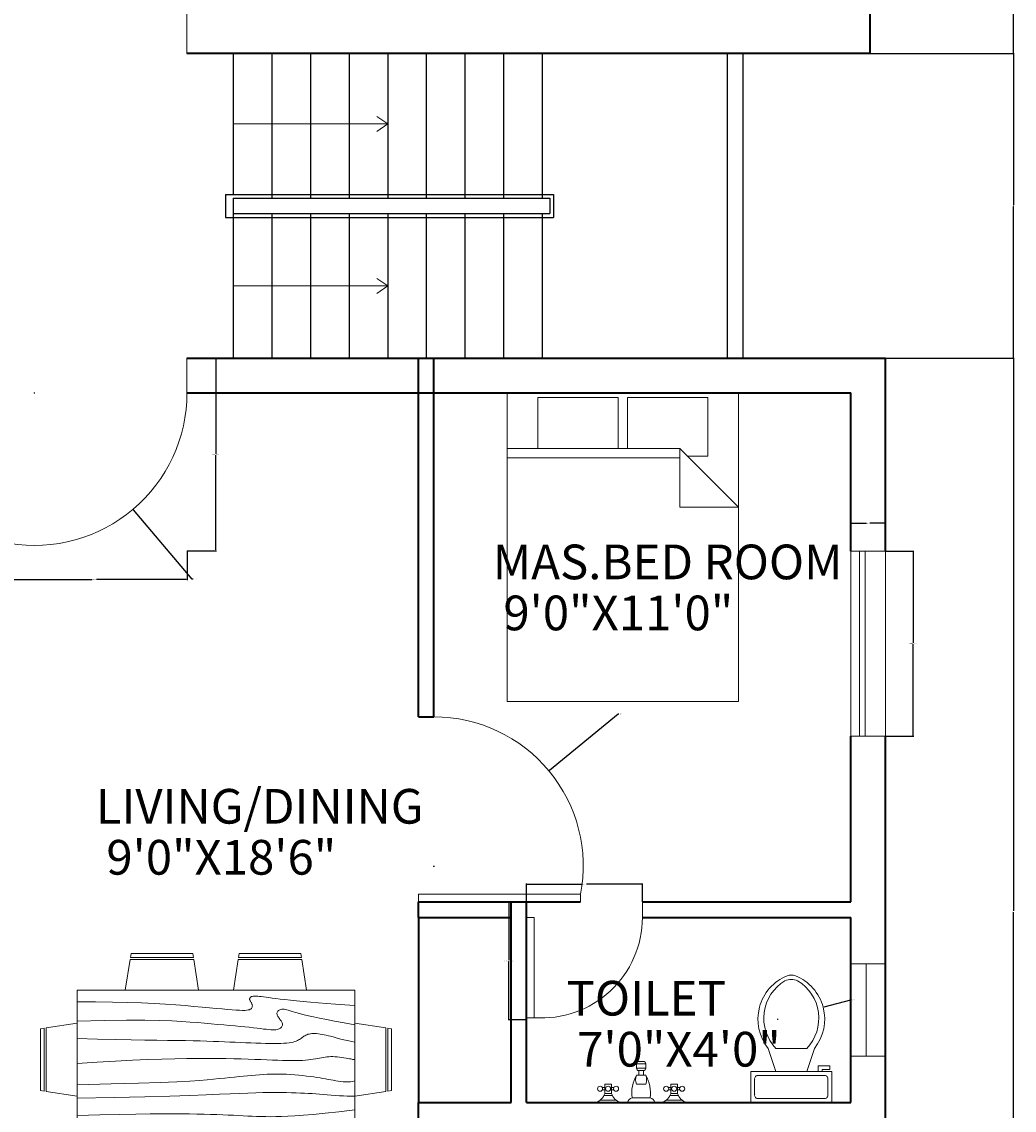
# Model space of a CAD drawing. Units: inches. Extents: x 2220 to 3422, y 783 to 1748.
# Tile 3 of 7: x 2483 to 2740, y 1023 to 1306. Entities that reach past the tile are written whole.
import ezdxf

# ---------------------------------------------------------------- set-up
doc = ezdxf.new("R2010")
doc.units = ezdxf.units.IN
for name, color, linetype, lineweight in [('A-ANNO-DIMS', 2, 'Continuous', 18), ('A-ANNO-SYMB', 2, 'Continuous', 18), ('A-AREA-IDEN', 7, 'Continuous', 18), ('A-DOOR', 3, 'Continuous', 20), ('A-FLOR-FIXT', 9, 'Continuous', 18), ('A-FLOR-STRS', 7, 'Continuous', 25), ('A-FURN', 8, 'Continuous', 18), ('A-GLAZ', 4, 'Continuous', 18), ('A-WALL', 7, 'Continuous', 40)]:
    doc.layers.add(name, color=color, linetype=linetype, lineweight=lineweight)
doc.styles.get("Standard").update_dxf_attribs({"font": 'arial.ttf'})
doc.dimstyles.get("Standard").update_dxf_attribs({"dimtxt": 0.18, "dimasz": 0.18, "dimexe": 0.18, "dimexo": 0.0625, "dimgap": 0.09, "dimtad": 0, "dimtih": 1, "dimtoh": 1, "dimdec": 4, "dimzin": 0, "dimdsep": 46, "dimtxsty": 'Standard', "dimcen": 0.09, "dimadec": 0, "dimazin": 0, "dimtfac": 1, "dimtdec": 4, "dimtofl": 0, "dimtmove": 0, "dimatfit": 3, "dimfxl": 1, "dimtolj": 1, "dimtzin": 0, "dimarcsym": 0})

# ---------------------------------------------------------------- blocks, each defined once
blk = doc.blocks.new('Bed - Queen')
for p, q in [((0, -80.00003), (0, 0)), ((0, 0), (59.99999, 0)), ((59.99999, 0), (59.99999, -80.00003)), ((7.99999, -1.2), (28.79998, -1.2)), ((7.99999, -14.4), (7.99999, -1.2)), ((28.79998, -1.2), (28.79998, -14.4)), ((31.19999, -1.2), (51.99999, -1.2)), ((31.19999, -14.4), (31.19999, -1.2)), ((51.99999, -1.2), (51.99999, -16.4)), ((0, -14.4), (44.8, -14.4)), ((44.8, -16.8), (0, -16.8)), ((59.99999, -29.6), (44.8, -14.4)), ((44.8, -14.4), (44.8, -29.6)), ((51.99999, -16.4), (46.79936, -16.4)), ((44.8, -29.6), (59.99999, -29.6)), ((59.99999, -80.00003), (0, -80.00003))]:
    blk.add_line(p, q)
blk = doc.blocks.new('Dining Set - 36 x 72 in.')
for p, q in [((-22.2343, 26.00059), (-23.4847, 17.99762)), ((-22.2304, 26), (-5.7608, 26)), ((-22, 27.5), (-22.1562, 26.50042)), ((-5.8416, 26.5), (-22.1534, 26.5)), ((-22, 27.5), (-6, 27.5)), ((-5.8437, 26.49966), (-6, 27.5)), ((-4.5152, 17.99762), (-5.7655, 25.99926)), ((5.7657, 26.00059), (4.5153, 17.99762)), ((5.7696, 26), (22.2392, 26)), ((6, 27.5), (5.8438, 26.50042)), ((22.1584, 26.5), (5.8466, 26.5)), ((6, 27.5), (22, 27.5)), ((22.1563, 26.49966), (22, 27.5)), ((23.4848, 17.99762), (22.2345, 25.99926)), ((36, 18), (-36, 18)), ((-36, 18), (-36, -18)), ((36, -18), (36, 18)), ((-44.0006, 8.23428), (-35.9976, 9.48474)), ((44.0006, 8.23428), (35.9976, 9.48474)), ((-45.5, 8), (-44.5004, 8.15617)), ((-45.5, 8), (-45.5, -8)), ((-44.5, -8.15843), (-44.5, 8.15338)), ((-44, 8.23041), (-44, -8.23915)), ((44, 8.23041), (44, -8.23915)), ((44.5, -8.15843), (44.5, 8.15338)), ((45.5, 8), (44.5005, 8.15617)), ((45.5, 8), (45.5, -8)), ((-44.4997, -8.15631), (-45.5, -8)), ((-35.9976, -9.48476), (-43.9993, -8.2345)), ((35.9976, -9.48476), (43.9993, -8.2345)), ((44.4997, -8.15631), (45.5, -8)), ((-36, -18), (36, -18)), ((-22.2343, -26.0006), (-23.4847, -17.99762)), ((-4.5152, -17.99762), (-5.7655, -25.99928)), ((5.7657, -26.0006), (4.5153, -17.99762)), ((23.4848, -17.99762), (22.2345, -25.99928)), ((-22.2304, -26), (-5.7608, -26)), ((-22, -27.5), (-22.1562, -26.50044)), ((-5.8416, -26.5), (-22.1534, -26.5)), ((-22, -27.5), (-6, -27.5)), ((-5.8437, -26.49967), (-6, -27.5)), ((5.7696, -26), (22.2392, -26)), ((6, -27.5), (5.8438, -26.50044)), ((22.1584, -26.5), (5.8466, -26.5)), ((6, -27.5), (22, -27.5)), ((22.1563, -26.49967), (22, -27.5))]:
    blk.add_line(p, q)
for points in [[(-36, 15), (-31.1772, 14.97754), (-26.8079, 14.91406), (-22.8538, 14.81543), (-19.276, 14.6875), (-16.0362, 14.53613), (-13.0957, 14.36718), (-10.4159, 14.18652), (-7.9583, 14), (-5.6904, 13.81315), (-3.6035, 13.63021), (-1.6954, 13.45508), (0.0365, 13.29166), (1.5945, 13.14388), (2.9811, 13.01562), (4.1988, 12.9108), (5.25, 12.83333), (6.1393, 12.78613), (6.8802, 12.76823), (7.4883, 12.77767), (7.9792, 12.8125), (8.3685, 12.87077), (8.6719, 12.95052), (8.9049, 13.0498), (9.0833, 13.16666), (9.2205, 13.29899), (9.3216, 13.44401), (9.3895, 13.59879), (9.4271, 13.76041), (9.4373, 13.92594), (9.4232, 14.09245), (9.3875, 14.257), (9.3333, 14.41666), (9.2638, 14.56917), (9.1836, 14.71484), (9.0975, 14.85465), (9.0104, 14.98958), (8.9272, 15.1206), (8.8529, 15.2487), (8.7922, 15.37483), (8.75, 15.5), (8.7305, 15.62467), (8.7344, 15.74739), (8.7617, 15.86621), (8.8125, 15.97916), (8.8867, 16.08431), (8.9844, 16.17968), (9.1055, 16.26334), (9.25, 16.33333), (9.4189, 16.38802), (9.6172, 16.42708), (9.8506, 16.45052), (10.125, 16.45833), (10.4463, 16.45052), (10.8203, 16.42708), (11.2529, 16.38802), (11.75, 16.33333), (12.3184, 16.26318), (12.9694, 16.17838), (13.7151, 16.07991), (14.5677, 15.96875), (15.5395, 15.84586), (16.6426, 15.71224), (17.8893, 15.56884), (19.2917, 15.41666), (20.859, 15.25667), (22.5879, 15.08984), (24.4721, 14.91715), (26.5052, 14.73958), (28.6809, 14.5581), (30.9929, 14.3737), (33.4347, 14.18733), (36, 14)], [(-36, 10), (-28.9766, 10.14274), (-23.1725, 10.20442), (-18.4241, 10.19775), (-14.5677, 10.13541), (-11.4399, 10.03011), (-8.877, 9.89453), (-6.7154, 9.74137), (-4.7917, 9.58333), (-2.9698, 9.43082), (-1.2246, 9.28515), (0.4415, 9.14534), (2.026, 9.01041), (3.5266, 8.87939), (4.9408, 8.7513), (6.266, 8.62516), (7.5, 8.5), (8.6411, 8.37549), (9.6914, 8.2539), (10.6538, 8.13818), (11.5312, 8.03125), (12.3267, 7.93603), (13.043, 7.85547), (13.6831, 7.79248), (14.25, 7.75), (14.7471, 7.7303), (15.1797, 7.73307), (15.5537, 7.75732), (15.875, 7.80208), (16.1494, 7.86637), (16.3828, 7.94922), (16.5811, 8.04964), (16.75, 8.16666), (16.8944, 8.29915), (17.0143, 8.44531), (17.1089, 8.60319), (17.1771, 8.77083), (17.218, 8.94629), (17.2305, 9.1276), (17.2137, 9.31282), (17.1667, 9.5), (17.0895, 9.6875), (16.987, 9.875), (16.8649, 10.0625), (16.7292, 10.25), (16.5856, 10.4375), (16.4401, 10.625), (16.2985, 10.8125), (16.1667, 11), (16.05, 11.18733), (15.9518, 11.3737), (15.8752, 11.5581), (15.8229, 11.73958), (15.798, 11.91715), (15.8034, 12.08984), (15.842, 12.25667), (15.9167, 12.41666), (16.0295, 12.56836), (16.1784, 12.70833), (16.3605, 12.83268), (16.5729, 12.9375), (16.8127, 13.01888), (17.0768, 13.07291), (17.3625, 13.0957), (17.6667, 13.08333), (17.9894, 13.03312), (18.3418, 12.94726), (18.7382, 12.82918), (19.1927, 12.68229), (19.7195, 12.51001), (20.3327, 12.31575), (21.0465, 12.10294), (21.875, 11.875), (22.8357, 11.63354), (23.959, 11.37304), (25.2786, 11.08618), (26.8282, 10.76562), (28.6414, 10.40405), (30.752, 9.99414), (33.1936, 9.52856), (36, 9)], [(-36, 5.5), (-30.7157, 5.3348), (-26.069, 5.20963), (-21.9946, 5.11767), (-18.4271, 5.05208), (-15.3009, 5.00602), (-12.5508, 4.97265), (-10.1112, 4.94515), (-7.9167, 4.91666), (-5.909, 4.88167), (-4.0586, 4.83984), (-2.3429, 4.79215), (-0.7396, 4.73958), (0.7739, 4.6831), (2.22, 4.6237), (3.6213, 4.56233), (5, 4.5), (6.373, 4.43782), (7.7344, 4.3776), (9.0723, 4.32129), (10.375, 4.27083), (11.6309, 4.22819), (12.8281, 4.19531), (13.9551, 4.17415), (15, 4.16666), (15.954, 4.17448), (16.819, 4.19791), (17.6001, 4.23698), (18.3021, 4.29166), (18.9299, 4.36198), (19.4883, 4.44791), (19.9823, 4.54948), (20.4167, 4.66666), (20.7969, 4.79899), (21.1302, 4.94401), (21.4245, 5.09879), (21.6875, 5.26041), (21.9271, 5.42594), (22.1511, 5.59245), (22.3672, 5.757), (22.5834, 5.91666), (22.8065, 6.06868), (23.0404, 6.21093), (23.2879, 6.34147), (23.5521, 6.45833), (23.8358, 6.55957), (24.142, 6.64323), (24.4735, 6.70735), (24.8334, 6.75), (25.2235, 6.76969), (25.642, 6.76692), (26.0858, 6.74267), (26.5521, 6.69791), (27.0379, 6.63362), (27.5404, 6.55078), (28.0565, 6.45036), (28.5834, 6.33333), (29.1242, 6.19987), (29.7071, 6.04687), (30.3661, 5.87044), (31.1354, 5.66666), (32.0493, 5.43164), (33.142, 5.16146), (34.4475, 4.85221), (36, 4.5)], [(-36, -1), (-30.7915, -0.6591), (-26.0195, -0.38216), (-21.6519, -0.16284), (-17.6563, 0.00521), (-14.0005, 0.12833), (-10.6523, 0.21289), (-7.5796, 0.26522), (-4.75, 0.29166), (-2.134, 0.29793), (0.2878, 0.28711), (2.5317, 0.26163), (4.6146, 0.22396), (6.5529, 0.17651), (8.3633, 0.12174), (10.0623, 0.06209), (11.6667, 0), (13.1899, -0.06201), (14.6341, -0.1211), (15.9982, -0.17432), (17.2813, -0.21875), (18.4823, -0.25147), (19.6003, -0.26953), (20.6343, -0.27002), (21.5834, -0.25), (22.4481, -0.20768), (23.2357, -0.14584), (23.9549, -0.06836), (24.6146, 0.02083), (25.2235, 0.11784), (25.7904, 0.21875), (26.3241, 0.31966), (26.8334, 0.41666), (27.3265, 0.50618), (27.8099, 0.58593), (28.2894, 0.65397), (28.7709, 0.70833), (29.2601, 0.74707), (29.763, 0.76823), (30.2855, 0.76985), (30.8334, 0.75), (31.4088, 0.70784), (31.9994, 0.64713), (32.589, 0.57275), (33.1615, 0.48958), (33.7008, 0.4025), (34.1908, 0.3164), (34.6153, 0.23616), (34.9584, 0.16666), (35.2099, 0.11165), (35.3848, 0.07031), (35.504, 0.04069), (35.5886, 0.02083), (35.6594, 0.00879), (35.7377, 0.0026), (35.8442, 0.00032), (36, 0)], [(-36, -6.5), (-27.1843, -6.31267), (-20.084, -6.1263), (-14.469, -5.9419), (-10.1094, -5.76042), (-6.7752, -5.58285), (-4.2363, -5.41016), (-2.2629, -5.24333), (-0.625, -5.08334), (0.8708, -4.93099), (2.2715, -4.78646), (3.5872, -4.64974), (4.8281, -4.52084), (6.0046, -4.39974), (7.127, -4.28646), (8.2053, -4.18099), (9.25, -4.08334), (10.2705, -3.99382), (11.2734, -3.91407), (12.2647, -3.84603), (13.25, -3.79167), (14.2354, -3.75293), (15.2266, -3.73177), (16.2295, -3.73015), (17.25, -3.75), (18.2912, -3.79248), (19.3451, -3.85547), (20.4009, -3.93604), (21.4479, -4.03125), (22.4754, -4.13819), (23.4727, -4.25391), (24.4289, -4.37549), (25.3334, -4.5), (26.1785, -4.62492), (26.9694, -4.74935), (27.7145, -4.87281), (28.4219, -4.99479), (29.1, -5.11483), (29.7572, -5.23242), (30.4016, -5.34709), (31.0417, -5.45834), (31.6837, -5.56437), (32.3262, -5.65821), (32.9658, -5.73153), (33.599, -5.77604), (34.2224, -5.78345), (34.8327, -5.74545), (35.4264, -5.65373), (36, -5.5)], [(-36, -10), (-26.4022, -9.81299), (-18.4675, -9.62891), (-11.9839, -9.45069), (-6.7396, -9.28125), (-2.5226, -9.12354), (0.8789, -8.98047), (3.6769, -8.85498), (6.0833, -8.75), (8.2767, -8.66765), (10.3021, -8.60677), (12.1712, -8.56543), (13.8958, -8.54167), (15.4876, -8.53353), (16.9583, -8.53907), (18.3197, -8.55632), (19.5834, -8.58334), (20.7616, -8.61841), (21.8685, -8.66081), (22.9188, -8.71004), (23.9271, -8.76563), (24.9081, -8.82707), (25.8763, -8.89388), (26.8465, -8.96558), (27.8334, -9.04167), (28.8474, -9.12118), (29.8828, -9.20117), (30.93, -9.27824), (31.9792, -9.34896), (33.0205, -9.40991), (34.0443, -9.45768), (35.0407, -9.48885), (36, -9.5)], [(-36, -14.5), (-30.0881, -14.33513), (-25.0332, -14.21224), (-20.7312, -14.12647), (-17.0781, -14.07292), (-13.97, -14.04671), (-11.3027, -14.04297), (-8.9724, -14.05681), (-6.875, -14.08334), (-4.9224, -14.11833), (-3.0905, -14.16016), (-1.3709, -14.20785), (0.2448, -14.26042), (1.7647, -14.3169), (3.1973, -14.3763), (4.5507, -14.43767), (5.8333, -14.5), (7.0554, -14.5621), (8.235, -14.62175), (9.3922, -14.67652), (10.5469, -14.72396), (11.7192, -14.76164), (12.929, -14.78711), (14.1965, -14.79794), (15.5417, -14.79167), (16.9933, -14.76424), (18.6152, -14.70508), (20.4804, -14.60197), (22.6615, -14.44271), (25.2312, -14.21509), (28.2624, -13.9069), (31.8277, -13.50594), (36, -13)]]:
    blk.add_lwpolyline(points)
blk = doc.blocks.new('Toilet - top')
for p, q in [((9.5, -6), (9.5, -2)), ((-8, -8.5), (-8, -8)), ((-7, -8), (-7, -9.5)), ((-4, -8), (-6, -14)), ((4, -8), (6, -14)), ((-10, -8.5), (-8, -8.5)), ((-10, -9.5), (-10, -8.5)), ((-7, -9.5), (-10, -9.5)), ((4, -14), (-4, -14))]:
    blk.add_line(p, q)
blk.add_lwpolyline([(10.5, -8), (10.5, 0), (-10.5, 0), (-10.5, -8)], close=True)
for points in [[(-9.5, -2), (-9.5, -6)], [(8.5, -1), (-8.5, -1)], [(-8.5, -7), (8.5, -7)]]:
    blk.add_lwpolyline(points)
for centre, radius, start, end in [((-8.62, -1.88), 0.884, 81.8699, 188.1301), ((8.62, -1.88), 0.884, 351.8699, 98.1301), ((-8.62, -6.12), 0.884, 171.8699, 278.1301), ((8.62, -6.12), 0.884, 261.8699, 8.1301), ((3.52, -21.58), 12.17, 141.4691, 247.9714), ((4.2, -21.82), 11.33, 136.3677, 238.9468), ((-3.52, -21.58), 12.17, 292.0284, 38.5307), ((-4.2, -21.82), 11.33, 301.053, 43.6321), ((0, -27.88), 4, 245.7318, 294.2682), ((0, -29), 4, 254.8605, 285.1395)]:
    blk.add_arc(centre, radius, start, end)
blk = doc.blocks.new('Faucet - Bathroom front')
for p, q in [((-0.5, 4.25), (0.5, 4.25)), ((0.5, 3.75), (-0.5, 3.75)), ((-0.5, 3), (0.5, 3)), ((-0.25, 3), (-0.25, 3.5)), ((0.25, 3.5), (0.25, 3)), ((-4, 1.625), (-4.25, 1.625)), ((-4, 1.375), (-4.25, 1.375)), ((-3.25, 1.625), (-3, 1.625)), ((-3.25, 1.375), (-3, 1.375)), ((0.5, 2), (-0.5, 2)), ((3.25, 1.625), (3, 1.625)), ((3.25, 1.375), (3, 1.375)), ((4, 1.625), (4.25, 1.625)), ((4, 1.375), (4.25, 1.375)), ((-5, 0), (-2.25, 0)), ((-4.5087, 0.25), (-2.7408, 0.25)), ((-3.1442, 0.75), (-4.0979, 0.75)), ((-1.5, 0), (1.5, 0)), ((-1, 0.5), (1, 0.5)), ((2.25, 0), (5, 0)), ((2.7413, 0.25), (4.5092, 0.25)), ((4.1058, 0.75), (3.1521, 0.75))]:
    blk.add_line(p, q)
for points in [[(-0.5, 3.75), (-0.5, 4.25)], [(-0.25, 4.5), (0.25, 4.5)], [(0.5, 4.25), (0.5, 3.75)], [(0.25, 3.5), (-0.25, 3.5)]]:
    blk.add_lwpolyline(points)
for points in [[(-4, 1), (-4, 2), (-3.25, 2), (-3.25, 1)], [(3.25, 1), (3.25, 2), (4, 2), (4, 1)]]:
    blk.add_lwpolyline(points, close=True)
for centre in [(-4.5, 1.5), (-3.625, 1.5), (-2.75, 1.5), (2.75, 1.5), (3.625, 1.5), (4.5, 1.5)]:
    blk.add_circle(centre, 0.2795)
for centre, radius, start, end in [((-0.2575, 4.2575), 0.2426, 88.22243, 181.7776), ((-0.2575, 3.7425), 0.2426, 178.2224, 271.7776), ((0.2575, 4.2575), 0.2426, 358.2224, 91.77757), ((0.2575, 3.7425), 0.2426, 268.2224, 1.777565), ((3, 1), 4.0311, 150.2551, 187.125), ((0.6413, 2.5), 1.246, 156.3417, 203.6583), ((-3, 1), 4.0311, 352.875, 29.74488), ((-0.6413, 2.5), 1.246, 336.3417, 23.65835), ((-5.375, 1.375), 1.4252, 285.2551, 344.7449), ((-1.875, 1.375), 1.4252, 195.2551, 254.7449), ((-0.7962, -0.2038), 0.7327, 106.1502, 163.8498), ((0.7962, -0.2038), 0.7327, 16.1502, 73.84979), ((1.875, 1.375), 1.4252, 285.2551, 344.7449), ((5.375, 1.375), 1.4252, 195.2551, 254.7449)]:
    blk.add_arc(centre, radius, start, end)
blk = doc.blocks.new('DOOR-UNIT-ENTRY')
for p, q in [((0, 48.53), (2, 48.53)), ((2, 0.53), (2, 48.53)), ((48, 39.53), (48, 48.53)), ((0, 39.53), (2, 39.53)), ((0, 0.53), (2, 0.53))]:
    blk.add_line(p, q)
blk.add_arc((8.47, 39.53), 39.53, 260.5843, 0)
blk = doc.blocks.new('DOOR-BATH-SWING')
for p, q in [((30, 26.06), (30, 30.06)), ((0, 26.06), (2, 26.06)), ((2, 0.06), (2, 26.06)), ((0, 0.06), (2, 0.06))]:
    blk.add_line(p, q)
blk.add_arc((3.93, 26.06), 26.07, 265.7578, 0)
blk = doc.blocks.new('WIN-48-OFFSET-A')
for p, q in [((0, 0), (0, 9)), ((0, 9), (48, 9)), ((48, 0), (48, 9)), ((0, 6.75), (48, 6.75)), ((0, 5.25), (48, 5.25)), ((0, 0), (48, 0))]:
    blk.add_line(p, q)
blk = doc.blocks.new('VENT-24-SINGLE')
for p, q in [((0, 24), (9, 24)), ((0, 24), (0, 0)), ((4, 0), (4, 24)), ((9, 24), (9, 0)), ((0, 0), (9, 0))]:
    blk.add_line(p, q)
blk = doc.blocks.new('ARROW-STAIR-DIRECTION')
for p, q in [((40, 1.95), (37.21, 3.9)), ((0, 1.95), (40, 1.95)), ((40, 1.95), (37.21, 0))]:
    blk.add_line(p, q)
blk = doc.blocks.new('*D25')
at = {"layer": 'A-ANNO-DIMS', "color": 0, "lineweight": -2, "transparency": 16777216}
for p, q in [((2706.61, 1168.39), (2713.93, 1168.39)), ((2713.75, 1168.21), (2713.75, 1144.57)), ((2713.75, 1120.57), (2713.75, 1144.21)), ((2706.61, 1120.39), (2713.93, 1120.39))]:
    blk.add_line(p, q, dxfattribs=at)
at = {"layer": 'A-ANNO-DIMS', "color": 0, "transparency": 16777216}
for points in [[(2713.72, 1168.21), (2713.78, 1168.21), (2713.75, 1168.39)], [(2713.72, 1120.57), (2713.78, 1120.57), (2713.75, 1120.39)]]:
    blk.add_solid(points, dxfattribs=at)
at = {"layer": 'Defpoints', "color": 0, "transparency": 16777216}
for p in [(2706.55, 1168.39), (2713.75, 1168.39), (2706.55, 1120.39)]:
    blk.add_point(p, dxfattribs=at)
at = {"layer": 'A-ANNO-DIMS', "color": 0, "transparency": 16777216, "insert": (2713.75, 1144.39), "char_height": 0.18, "attachment_point": 5}
blk.add_mtext('\\A1;WINDOW A 48 TYP.', dxfattribs=at)
blk = doc.blocks.new('*D26')
at = {"layer": 'A-ANNO-DIMS', "color": 0, "lineweight": -2, "transparency": 16777216}
for p, q in [((2697.55, 1168.45), (2697.55, 1175.77)), ((2697.73, 1175.59), (2701.59, 1175.59)), ((2706.37, 1175.59), (2702.5, 1175.59)), ((2706.55, 1168.45), (2706.55, 1175.77))]:
    blk.add_line(p, q, dxfattribs=at)
at = {"layer": 'A-ANNO-DIMS', "color": 0, "transparency": 16777216}
for points in [[(2697.73, 1175.62), (2697.73, 1175.56), (2697.55, 1175.59)], [(2706.37, 1175.62), (2706.37, 1175.56), (2706.55, 1175.59)]]:
    blk.add_solid(points, dxfattribs=at)
at = {"layer": 'Defpoints', "color": 0, "transparency": 16777216}
for p in [(2697.55, 1175.59), (2697.55, 1168.39), (2706.55, 1168.39)]:
    blk.add_point(p, dxfattribs=at)
at = {"layer": 'A-ANNO-DIMS', "color": 0, "transparency": 16777216, "insert": (2702.05, 1175.59), "char_height": 0.18, "attachment_point": 5}
blk.add_mtext('\\A1;9 TYP.', dxfattribs=at)
blk = doc.blocks.new('*D39')
at = {"layer": 'A-ANNO-DIMS', "color": 0, "lineweight": -2, "transparency": 16777216}
for p, q in [((2525.61, 1218.39), (2533.21, 1218.39)), ((2533.03, 1218.21), (2533.03, 1193.62)), ((2533.03, 1168.67), (2533.03, 1193.26)), ((2525.61, 1168.49), (2533.21, 1168.49))]:
    blk.add_line(p, q, dxfattribs=at)
at = {"layer": 'A-ANNO-DIMS', "color": 0, "transparency": 16777216}
for points in [[(2533, 1218.21), (2533.06, 1218.21), (2533.03, 1218.39)], [(2533, 1168.67), (2533.06, 1168.67), (2533.03, 1168.49)]]:
    blk.add_solid(points, dxfattribs=at)
at = {"layer": 'Defpoints', "color": 0, "transparency": 16777216}
for p in [(2525.55, 1218.39), (2533.03, 1218.39), (2525.55, 1168.49)]:
    blk.add_point(p, dxfattribs=at)
at = {"layer": 'A-ANNO-DIMS', "color": 0, "transparency": 16777216, "insert": (2533.03, 1193.44), "char_height": 0.18, "attachment_point": 5}
blk.add_mtext('\\A1;ENTRY 50 TYP.', dxfattribs=at)
blk = doc.blocks.new('*D40')
at = {"layer": 'A-ANNO-DIMS', "color": 0, "lineweight": -2, "transparency": 16777216}
for p, q in [((2477.55, 1168.43), (2477.55, 1160.83)), ((2525.55, 1168.43), (2525.55, 1160.83)), ((2477.73, 1161.01), (2501.01, 1161.01)), ((2525.37, 1161.01), (2502.08, 1161.01))]:
    blk.add_line(p, q, dxfattribs=at)
at = {"layer": 'A-ANNO-DIMS', "color": 0, "transparency": 16777216}
for points in [[(2477.73, 1161.04), (2477.73, 1160.98), (2477.55, 1161.01)], [(2525.37, 1161.04), (2525.37, 1160.98), (2525.55, 1161.01)]]:
    blk.add_solid(points, dxfattribs=at)
at = {"layer": 'Defpoints', "color": 0, "transparency": 16777216}
for p in [(2477.55, 1168.49), (2525.55, 1168.49), (2525.55, 1161.01)]:
    blk.add_point(p, dxfattribs=at)
at = {"layer": 'A-ANNO-DIMS', "color": 0, "transparency": 16777216, "insert": (2501.55, 1161.01), "char_height": 0.18, "attachment_point": 5}
blk.add_mtext('\\A1;48 TYP.', dxfattribs=at)
blk = doc.blocks.new('*D41')
at = {"layer": 'A-ANNO-DIMS', "color": 0, "lineweight": -2, "transparency": 16777216}
for p, q in [((2613.48, 1077.39), (2608.79, 1077.39)), ((2608.97, 1077.21), (2608.97, 1062.31)), ((2608.97, 1047.03), (2608.97, 1061.94)), ((2613.48, 1046.85), (2608.79, 1046.85))]:
    blk.add_line(p, q, dxfattribs=at)
at = {"layer": 'A-ANNO-DIMS', "color": 0, "transparency": 16777216}
for points in [[(2608.94, 1077.21), (2609, 1077.21), (2608.97, 1077.39)], [(2608.94, 1047.03), (2609, 1047.03), (2608.97, 1046.85)]]:
    blk.add_solid(points, dxfattribs=at)
at = {"layer": 'Defpoints', "color": 0, "transparency": 16777216}
for p in [(2608.97, 1077.39), (2613.55, 1077.39), (2613.55, 1046.85)]:
    blk.add_point(p, dxfattribs=at)
at = {"layer": 'A-ANNO-DIMS', "color": 0, "transparency": 16777216, "insert": (2608.97, 1062.12), "char_height": 0.18, "attachment_point": 5}
blk.add_mtext('\\A1;BATH DOOR 31 TYP.', dxfattribs=at)
blk = doc.blocks.new('*D42')
at = {"layer": 'A-ANNO-DIMS', "color": 0, "lineweight": -2, "transparency": 16777216}
for p, q in [((2613.55, 1077.45), (2613.55, 1082.15)), ((2613.73, 1081.97), (2628.02, 1081.97)), ((2643.37, 1081.97), (2629.07, 1081.97)), ((2643.55, 1077.45), (2643.55, 1082.15))]:
    blk.add_line(p, q, dxfattribs=at)
at = {"layer": 'A-ANNO-DIMS', "color": 0, "transparency": 16777216}
for points in [[(2613.73, 1082), (2613.73, 1081.94), (2613.55, 1081.97)], [(2643.37, 1082), (2643.37, 1081.94), (2643.55, 1081.97)]]:
    blk.add_solid(points, dxfattribs=at)
at = {"layer": 'Defpoints', "color": 0, "transparency": 16777216}
for p in [(2643.55, 1081.97), (2613.55, 1077.39), (2643.55, 1077.39)]:
    blk.add_point(p, dxfattribs=at)
at = {"layer": 'A-ANNO-DIMS', "color": 0, "transparency": 16777216, "insert": (2628.55, 1081.97), "char_height": 0.18, "attachment_point": 5}
blk.add_mtext('\\A1;30 TYP.', dxfattribs=at)
blk = doc.blocks.new('*D55')
at = {"layer": 'A-ANNO-DIMS', "color": 0, "lineweight": -2, "transparency": 16777216}
for p, q in [((2702.61, 1297.39), (2739.88, 1297.39)), ((2739.7, 1297.21), (2739.7, 1258.07)), ((2739.7, 1218.57), (2739.7, 1257.71)), ((2706.61, 1218.39), (2739.88, 1218.39))]:
    blk.add_line(p, q, dxfattribs=at)
at = {"layer": 'A-ANNO-DIMS', "color": 0, "transparency": 16777216}
for points in [[(2739.67, 1297.21), (2739.73, 1297.21), (2739.7, 1297.39)], [(2739.67, 1218.57), (2739.73, 1218.57), (2739.7, 1218.39)]]:
    blk.add_solid(points, dxfattribs=at)
at = {"layer": 'Defpoints', "color": 0, "transparency": 16777216}
for p in [(2702.55, 1297.39), (2706.55, 1218.39), (2739.7, 1218.39)]:
    blk.add_point(p, dxfattribs=at)
at = {"layer": 'A-ANNO-DIMS', "color": 0, "transparency": 16777216, "insert": (2739.7, 1257.89), "char_height": 0.18, "attachment_point": 5}
blk.add_mtext('\\A1;79', dxfattribs=at)
blk = doc.blocks.new('*D56')
at = {"layer": 'A-ANNO-DIMS', "color": 0, "lineweight": -2, "transparency": 16777216}
for p, q in [((2702.61, 1578.39), (2739.88, 1578.39)), ((2739.7, 1578.21), (2739.7, 1438.07)), ((2739.7, 1297.57), (2739.7, 1437.71)), ((2702.61, 1297.39), (2739.88, 1297.39))]:
    blk.add_line(p, q, dxfattribs=at)
at = {"layer": 'A-ANNO-DIMS', "color": 0, "transparency": 16777216}
for points in [[(2739.67, 1578.21), (2739.73, 1578.21), (2739.7, 1578.39)], [(2739.67, 1297.57), (2739.73, 1297.57), (2739.7, 1297.39)]]:
    blk.add_solid(points, dxfattribs=at)
at = {"layer": 'Defpoints', "color": 0, "transparency": 16777216}
for p in [(2702.55, 1578.39), (2739.7, 1578.39), (2702.55, 1297.39)]:
    blk.add_point(p, dxfattribs=at)
at = {"layer": 'A-ANNO-DIMS', "color": 0, "transparency": 16777216, "insert": (2739.7, 1437.89), "char_height": 0.18, "attachment_point": 5}
blk.add_mtext('\\A1;281', dxfattribs=at)
blk = doc.blocks.new('*D57')
at = {"layer": 'A-ANNO-DIMS', "color": 0, "lineweight": -2, "transparency": 16777216}
for p, q in [((2706.61, 1218.39), (2739.88, 1218.39)), ((2739.7, 1218.21), (2739.7, 1075.07)), ((2739.7, 931.57), (2739.7, 1074.71)), ((2706.61, 931.39), (2739.88, 931.39))]:
    blk.add_line(p, q, dxfattribs=at)
at = {"layer": 'A-ANNO-DIMS', "color": 0, "transparency": 16777216}
for points in [[(2739.67, 1218.21), (2739.73, 1218.21), (2739.7, 1218.39)], [(2739.67, 931.57), (2739.73, 931.57), (2739.7, 931.39)]]:
    blk.add_solid(points, dxfattribs=at)
at = {"layer": 'Defpoints', "color": 0, "transparency": 16777216}
for p in [(2706.55, 1218.39), (2706.55, 931.39), (2739.7, 931.39)]:
    blk.add_point(p, dxfattribs=at)
at = {"layer": 'A-ANNO-DIMS', "color": 0, "transparency": 16777216, "insert": (2739.7, 1074.89), "char_height": 0.18, "attachment_point": 5}
blk.add_mtext('\\A1;287', dxfattribs=at)
blk = doc.blocks.new('*D75')
at = {"layer": 'A-ANNO-DIMS', "color": 0, "lineweight": -2, "transparency": 16777216}
for p, q in [((2485.92, 1209.39), (2486.1, 1209.39)), ((2486.01, 1209.3), (2486.01, 1209.48)), ((2526.92, 1161.14), (2511.7, 1179.1)), ((2527.1, 1161.14), (2526.92, 1161.14))]:
    blk.add_line(p, q, dxfattribs=at)
at = {"layer": 'A-ANNO-DIMS', "color": 0, "transparency": 16777216}
blk.add_solid([(2511.72, 1179.12), (2511.67, 1179.08), (2511.58, 1179.24)], dxfattribs=at)
at = {"layer": 'Defpoints', "color": 0, "transparency": 16777216}
for p in [(2486.01, 1209.39), (2511.58, 1179.24)]:
    blk.add_point(p, dxfattribs=at)
at = {"layer": 'A-ANNO-DIMS', "color": 0, "transparency": 16777216, "insert": (2527.58, 1161.14), "char_height": 0.18, "attachment_point": 5}
blk.add_mtext('\\A1;R39.53', dxfattribs=at)
blk = doc.blocks.new('*D76')
at = {"layer": 'A-ANNO-DIMS', "color": 0, "lineweight": -2, "transparency": 16777216}
for p, q in [((2637.28, 1126.13), (2619.52, 1111.45)), ((2637.46, 1126.13), (2637.28, 1126.13)), ((2589.46, 1086.7), (2589.64, 1086.7)), ((2589.55, 1086.61), (2589.55, 1086.79))]:
    blk.add_line(p, q, dxfattribs=at)
at = {"layer": 'A-ANNO-DIMS', "color": 0, "transparency": 16777216}
blk.add_solid([(2619.5, 1111.48), (2619.54, 1111.43), (2619.38, 1111.34)], dxfattribs=at)
at = {"layer": 'Defpoints', "color": 0, "transparency": 16777216}
for p in [(2619.38, 1111.34), (2589.55, 1086.7)]:
    blk.add_point(p, dxfattribs=at)
at = {"layer": 'A-ANNO-DIMS', "color": 0, "transparency": 16777216, "insert": (2638.01, 1126.13), "char_height": 0.18, "attachment_point": 5}
blk.add_mtext('\\A1;R38.696', dxfattribs=at)
blk = doc.blocks.new('*D88')
at = {"layer": 'A-ANNO-DIMS', "color": 0, "lineweight": -2, "transparency": 16777216}
for p, q in [((2697.45, 1051.94), (2690.57, 1050.13)), ((2678.53, 1046.99), (2678.71, 1046.99)), ((2678.62, 1046.9), (2678.62, 1047.08))]:
    blk.add_line(p, q, dxfattribs=at)
at = {"layer": 'A-ANNO-DIMS', "color": 0, "transparency": 16777216}
blk.add_solid([(2690.56, 1050.16), (2690.57, 1050.1), (2690.39, 1050.08)], dxfattribs=at)
at = {"layer": 'Defpoints', "color": 0, "transparency": 16777216}
for p in [(2690.39, 1050.08), (2678.62, 1046.99)]:
    blk.add_point(p, dxfattribs=at)
at = {"layer": 'A-ANNO-DIMS', "color": 0, "transparency": 16777216, "insert": (2698.13, 1051.94), "char_height": 0.18, "attachment_point": 5}
blk.add_mtext('\\A1;8X R12.17', dxfattribs=at)

msp = doc.modelspace()

# ---------------------------------------------------------------- linework, layer by layer
at = {"layer": 'A-DOOR'}
for p, q in [((2585.5466, 1077.3907), (2585.5466, 1079.3907)), ((2585.5466, 1079.3907), (2627.5466, 1079.3907)), ((2627.5466, 1077.3907), (2627.5466, 1079.3907))]:
    msp.add_line(p, q, dxfattribs=at)
msp.add_arc((2589.5466, 1086.695), 38.6957, 349.119336, 90, dxfattribs=at)
at = {"layer": 'A-FLOR-STRS'}
for p, q in [((2537.5466, 1297.3907), (2537.5466, 1260.8907)), ((2547.5466, 1297.3907), (2547.5466, 1259.8907)), ((2557.5466, 1297.3907), (2557.5466, 1259.8907)), ((2567.5466, 1297.3907), (2567.5466, 1259.8907)), ((2577.5466, 1297.3907), (2577.5466, 1259.8907)), ((2587.5466, 1297.3907), (2587.5466, 1259.8907)), ((2597.5466, 1297.3907), (2597.5466, 1259.8907)), ((2607.5466, 1297.3907), (2607.5466, 1259.8907)), ((2617.5466, 1297.3907), (2617.5466, 1259.8907)), ((2665.5466, 1297.3907), (2665.5466, 1218.3907)), ((2669.5466, 1297.3907), (2669.5466, 1218.3907)), ((2535.5466, 1260.8907), (2535.5466, 1254.8907)), ((2535.5466, 1260.8907), (2620.5466, 1260.8907)), ((2537.5466, 1259.8907), (2619.5466, 1259.8907)), ((2537.5466, 1259.8907), (2537.5466, 1218.3907)), ((2619.5466, 1259.8907), (2619.5466, 1255.8907)), ((2620.5466, 1260.8907), (2620.5466, 1254.8907)), ((2535.5466, 1254.8907), (2620.5466, 1254.8907)), ((2537.5466, 1255.8907), (2619.5466, 1255.8907)), ((2547.5466, 1255.8907), (2547.5466, 1218.3907)), ((2557.5466, 1255.8907), (2557.5466, 1218.3907)), ((2567.5466, 1255.8907), (2567.5466, 1218.3907)), ((2577.5466, 1255.8907), (2577.5466, 1218.3907)), ((2587.5466, 1255.8907), (2587.5466, 1218.3907)), ((2597.5466, 1255.8907), (2597.5466, 1218.3907)), ((2607.5466, 1255.8907), (2607.5466, 1218.3907)), ((2617.5466, 1255.8907), (2617.5466, 1218.3907))]:
    msp.add_line(p, q, dxfattribs=at)
at = {"layer": 'A-WALL'}
for p, q in [((2702.5466, 1297.3907), (2702.5466, 1403.3907)), ((2702.5466, 1297.3907), (2525.5466, 1297.3907)), ((2525.5466, 1218.3907), (2706.5466, 1218.3907)), ((2585.5466, 1125.3907), (2585.5466, 1218.3907)), ((2589.5466, 1125.3907), (2589.5466, 1218.3907)), ((2706.5466, 1168.3907), (2706.5466, 1218.3907)), ((2525.5466, 1209.3907), (2697.5466, 1209.3907)), ((2697.5466, 1168.3907), (2697.5466, 1209.3907)), ((2585.5466, 1125.3907), (2589.5466, 1125.3907)), ((2697.5466, 1077.3907), (2697.5466, 1120.3907)), ((2706.5466, 1037.3907), (2706.5466, 1120.3907)), ((2585.5466, 1077.3907), (2613.5466, 1077.3907)), ((2585.5466, 1073.3907), (2585.5466, 1077.3907)), ((2609.5466, 1025.3907), (2609.5466, 1077.3907)), ((2613.5466, 1025.3907), (2613.5466, 1077.3907)), ((2613.5466, 1077.3907), (2627.5466, 1077.3907)), ((2643.5466, 1077.3907), (2697.5466, 1077.3907)), ((2585.5466, 1073.3907), (2609.5466, 1073.3907)), ((2585.5466, 1073.3907), (2585.5466, 1025.3907)), ((2643.5466, 1073.3907), (2697.5466, 1073.3907)), ((2697.5466, 1037.3907), (2697.5466, 1073.3907)), ((2697.5466, 1025.3907), (2697.5466, 1037.3907)), ((2706.5466, 1000.8907), (2706.5466, 1037.3907)), ((2585.5466, 1021.3907), (2585.5466, 1025.3907)), ((2585.5466, 1025.3907), (2609.5466, 1025.3907)), ((2613.5466, 1025.3907), (2697.5466, 1025.3907))]:
    msp.add_line(p, q, dxfattribs=at)

# ---------------------------------------------------------------- block references
at = {"layer": 'A-ANNO-SYMB'}
for p in [(2537.547, 1277.192), (2537.547, 1235.192)]:
    msp.add_blockref('ARROW-STAIR-DIRECTION', p, dxfattribs=at)
at = {"layer": 'A-DOOR', "extrusion": (0, 0, -1), "zscale": -1, "rotation": 180}
msp.add_blockref('DOOR-UNIT-ENTRY', (-2477.547, 1345.9234), dxfattribs=at)
at = {"layer": 'A-DOOR'}
for name, p in [('DOOR-UNIT-ENTRY', (2477.547, 1169.858)), ('DOOR-BATH-SWING', (2613.547, 1047.326))]:
    msp.add_blockref(name, p, dxfattribs=at)
at = {"layer": 'A-FLOR-FIXT', "rotation": 180}
msp.add_blockref('Toilet - top', (2682.1427, 1025.4097), dxfattribs=at)
at = {"layer": 'A-FLOR-FIXT', "xscale": 2.361580970438625, "yscale": 2.361580970438625, "zscale": 2.361580970438625}
msp.add_blockref('Faucet - Bathroom front', (2643.2231, 1025.4097), dxfattribs=at)
at = {"layer": 'A-FURN'}
for name, p in [('Bed - Queen', (2608.4834, 1209.3907)), ('Dining Set - 36 x 72 in.', (2533.0492, 1036.5138))]:
    msp.add_blockref(name, p, dxfattribs=at)
at = {"layer": 'A-GLAZ', "rotation": 89.99999999999845}
msp.add_blockref('WIN-48-OFFSET-A', (2706.5463, 1120.3911), dxfattribs=at)
at = {"layer": 'A-GLAZ'}
msp.add_blockref('VENT-24-SINGLE', (2697.547, 1037.391), dxfattribs=at)

# ---------------------------------------------------------------- texts
at = {"layer": 'A-AREA-IDEN'}
for s, p in [('MAS.BED ROOM', (2604.7702, 1161.0724)), (' 9\'0"X11\'0"', (2604.7702, 1147.8454)), ('LIVING/DINING', (2501.8957, 1097.707)), (' 9\'0"X18\'6"', (2501.8957, 1084.4799)), ('TOILET', (2623.9005, 1047.9391)), (' 7\'0"X4\'0"', (2623.9005, 1034.7121))]:
    msp.add_text(s, height=9, dxfattribs=at).set_placement(p)

# ---------------------------------------------------------------- dimensions: what is measured, and where the dimension line sits
at = {"layer": 'A-ANNO-DIMS'}
for base, p1, p2, picture, middle in [((2739.6966, 1578.3907), (2702.5466, 1297.3907), (2702.5466, 1578.3907), '*D56', (2739.6966, 1437.8907)), ((2739.6966, 1218.3907), (2702.5466, 1297.3907), (2706.5466, 1218.3907), '*D55', (2739.6966, 1257.8907)), ((2739.6966, 931.3907), (2706.5466, 1218.3907), (2706.5466, 931.3907), '*D57', (2739.6966, 1074.8907))]:
    dim = msp.add_linear_dim(base=base, p1=p1, p2=p2, angle=90, dimstyle='Standard', override={"dimdec": 0, "dimlfac": 1, "dimrnd": 0, "dimzin": 0, "dimdsep": 46, "dimlunit": 2}, dxfattribs=at)
    dim.commit()
    dim.dimension.update_dxf_attribs({"geometry": picture, "text_midpoint": middle})
for base, p1, p2, angle, text, picture, middle in [((2533.0317, 1218.3907), (2525.5466, 1168.4905), (2525.5466, 1218.3907), 90, 'ENTRY <> TYP.', '*D39', (2533.0317, 1193.4406)), ((2697.5466, 1175.5907), (2706.5466, 1168.3907), (2697.5466, 1168.3907), 180, '<> TYP.', '*D26', (2702.0466, 1175.5907)), ((2713.7466, 1168.3907), (2706.5466, 1120.3907), (2706.5466, 1168.3907), 90, 'WINDOW A <> TYP.', '*D25', (2713.7466, 1144.3907)), ((2608.9662, 1077.3907), (2613.5466, 1046.8544), (2613.5466, 1077.3907), 90, 'BATH DOOR <> TYP.', '*D41', (2608.9662, 1062.1226))]:
    dim = msp.add_linear_dim(base=base, p1=p1, p2=p2, angle=angle, text=text, dimstyle='Standard', override={"dimdec": 0, "dimlfac": 1, "dimrnd": 0, "dimzin": 0, "dimdsep": 46, "dimlunit": 2}, dxfattribs=at)
    dim.commit()
    dim.dimension.update_dxf_attribs({"geometry": picture, "text_midpoint": middle})
for center, mpoint, override, picture, middle in [((2486.014, 1209.3907), (2511.5791, 1179.2369), {"dimdec": 2, "dimlfac": 1, "dimrnd": 0, "dimzin": 0, "dimdsep": 46, "dimlunit": 2}, '*D75', (2527.578, 1161.1446)), ((2589.5466, 1086.695), (2619.3795, 1111.3396), {"dimdec": 3, "dimlfac": 1, "dimrnd": 0, "dimzin": 0, "dimdsep": 46, "dimlunit": 2}, '*D76', (2638.0089, 1126.1263))]:
    dim = msp.add_radius_dim(center=center, mpoint=mpoint, dimstyle='Standard', override=override, dxfattribs=at)
    dim.commit()
    dim.dimension.update_dxf_attribs({"geometry": picture, "text_midpoint": middle, "dimtype": 164})
for base, p1, p2, picture, middle in [((2525.5466, 1161.0055), (2477.5466, 1168.4905), (2525.5466, 1168.4905), '*D40', (2501.5466, 1161.0055)), ((2643.5466, 1081.9711), (2613.5466, 1077.3907), (2643.5466, 1077.3907), '*D42', (2628.5466, 1081.9711))]:
    dim = msp.add_linear_dim(base=base, p1=p1, p2=p2, text='<> TYP.', dimstyle='Standard', override={"dimdec": 0, "dimlfac": 1, "dimrnd": 0, "dimzin": 0, "dimdsep": 46, "dimlunit": 2}, dxfattribs=at)
    dim.commit()
    dim.dimension.update_dxf_attribs({"geometry": picture, "text_midpoint": middle})
dim = msp.add_radius_dim(center=(2678.6231, 1046.9902), mpoint=(2690.3928, 1050.082), text='8X <>', dimstyle='Standard', override={"dimdec": 2, "dimlfac": 1, "dimrnd": 0, "dimzin": 0, "dimdsep": 46, "dimlunit": 2}, dxfattribs=at)
dim.commit()
dim.dimension.update_dxf_attribs({"geometry": '*D88', "text_midpoint": (2697.4547, 1051.937), "dimtype": 164})

doc.saveas('drawing.dxf')
